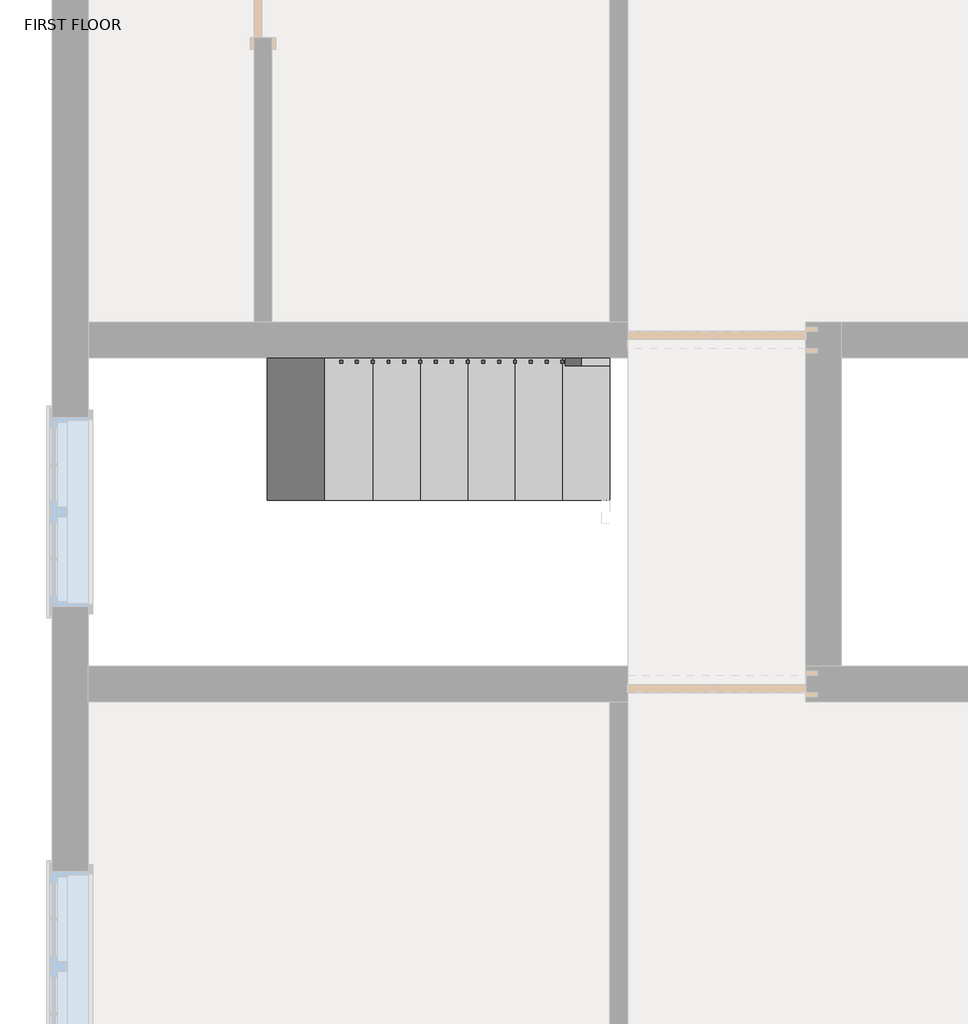
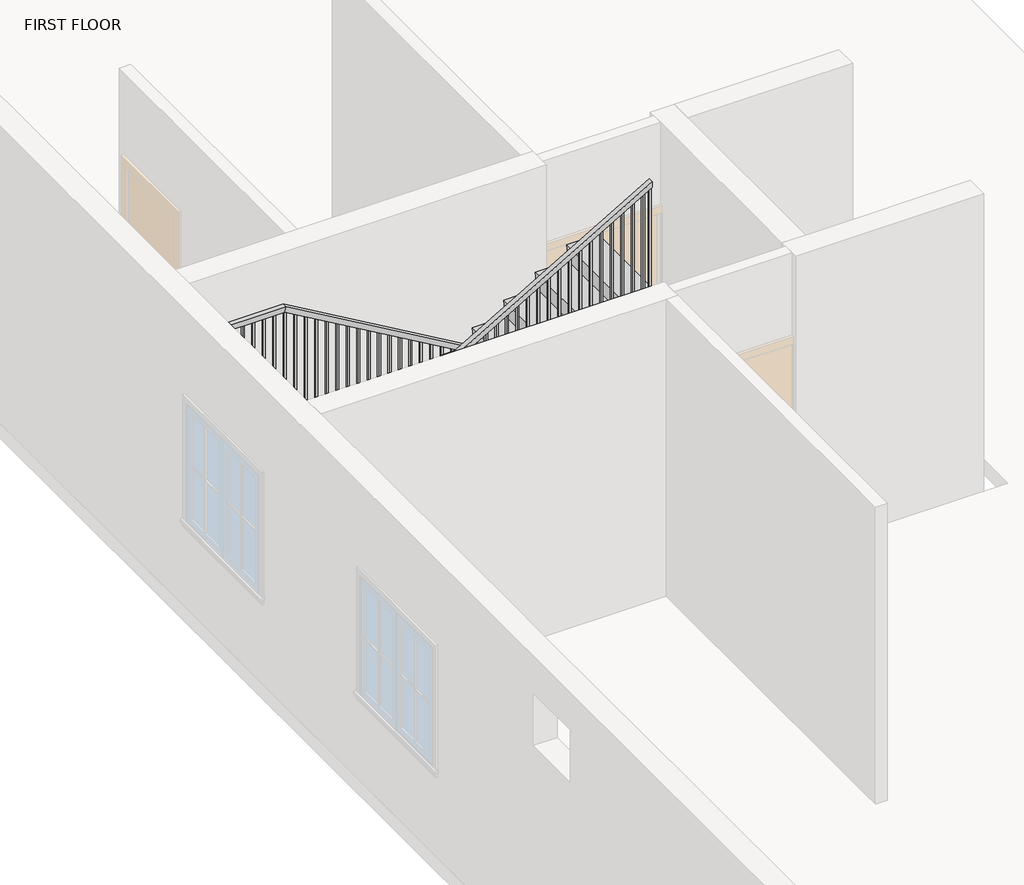
# One storey, part 3 of 4: 1 railing, 1 stair flight.
"""IFC4 building model written with IfcOpenShell, lengths in millimetres."""

from ifc_helpers import new_model, si_unit, frame, origin, place, context, project, spatial, polyline, outline, extrude, faceted_brep, element, save

model = new_model("IFC4")

# Units and contexts
model_context = context("Model", 3, world=origin())
ifc_project = project(units=[si_unit("LENGTHUNIT", "METRE", prefix="MILLI")], contexts=[model_context])

# Site, building, storey
site = spatial("IfcSite", under=ifc_project)
building = spatial("IfcBuilding", under=site)
storey = spatial("IfcBuildingStorey", under=building, Name="FIRST FLOOR", Elevation=3200.4)

# Railing
placement = place(None, origin())
element("IfcRailing", 1, ObjectType="Handrail - Rectangular", at=placement, inside=storey, context=model_context, shape_type="SolidModel", body=[
    faceted_brep([(-2776.8289041, 1499.0153263, 4292.6), (-2776.8289041, 1499.0153263, 4233.7886538), (-2776.8289041, 1549.8153263, 4233.7886538), (-2776.8289041, 1549.8153263, 4292.6), (-5215.2289041, 1499.0153263, 5715.0), (-5228.9626405, 1499.0153263, 5664.2), (-5228.9626405, 1549.8153263, 5664.2), (-5215.2289041, 1549.8153263, 5715.0), (-6078.8289041, 1499.0153263, 5715.0), (-6078.8289041, 1499.0153263, 5664.2), (-6129.6289041, 1549.8153263, 5664.2), (-6129.6289041, 1549.8153263, 5715.0), (-6078.8289041, -380.5846737, 5715.0), (-6078.8289041, -380.5846737, 5664.2), (-6129.6289041, -431.3846737, 5664.2), (-6129.6289041, -431.3846737, 5715.0), (-5520.0289041, -380.5846737, 5715.0), (-5506.2951677, -380.5846737, 5664.2), (-5506.2951677, -431.3846737, 5664.2), (-5520.0289041, -431.3846737, 5715.0), (-2776.8289041, -380.5846737, 7315.2), (-2776.8289041, -431.3846737, 7315.2), (-2776.8289041, -431.3846737, 7256.3886538), (-2776.8289041, -380.5846737, 7256.3886538)], [[[0, 1, 2, 3]], [[1, 0, 4, 5]], [[2, 1, 5, 6]], [[3, 2, 6, 7]], [[0, 3, 7, 4]], [[5, 4, 8, 9]], [[6, 5, 9, 10]], [[7, 6, 10, 11]], [[4, 7, 11, 8]], [[9, 8, 12, 13]], [[10, 9, 13, 14]], [[11, 10, 14, 15]], [[8, 11, 15, 12]], [[13, 12, 16, 17]], [[14, 13, 17, 18]], [[15, 14, 18, 19]], [[12, 15, 19, 16]], [[20, 21, 22, 23]], [[17, 16, 20, 23]], [[18, 17, 23, 22]], [[19, 18, 22, 21]], [[16, 19, 21, 20]]]),
    extrude(outline(polyline([(7217.4949038, -2843.5039041), (7206.3824038, -2862.5539041), (6223.0, -2862.5539041), (6223.0, -2843.5039041), (7217.4949038, -2843.5039041)])), frame((0.0, -415.5096737, 0.0), z_axis=(0.0, 1.0, 0.0), x_axis=(0.0, 0.0, 1.0)), (0.0, 0.0, 1.0), 19.05),
    extrude(outline(polyline([(7158.2282371, -2945.1039041), (7147.1157371, -2964.1539041), (6223.0, -2964.1539041), (6223.0, -2945.1039041), (7158.2282371, -2945.1039041)])), frame((0.0, -415.5096737, 0.0), z_axis=(0.0, 1.0, 0.0), x_axis=(0.0, 0.0, 1.0)), (0.0, 0.0, 1.0), 19.05),
    extrude(outline(polyline([(7098.9615704, -3046.7039041), (7087.8490704, -3065.7539041), (6223.0, -3065.7539041), (6223.0, -3046.7039041), (7098.9615704, -3046.7039041)])), frame((0.0, -415.5096737, 0.0), z_axis=(0.0, 1.0, 0.0), x_axis=(0.0, 0.0, 1.0)), (0.0, 0.0, 1.0), 19.05),
    extrude(outline(polyline([(7039.6949038, -3148.3039041), (7028.5824038, -3167.3539041), (6045.2, -3167.3539041), (6045.2, -3148.3039041), (7039.6949038, -3148.3039041)])), frame((0.0, -415.5096737, 0.0), z_axis=(0.0, 1.0, 0.0), x_axis=(0.0, 0.0, 1.0)), (0.0, 0.0, 1.0), 19.05),
    extrude(outline(polyline([(6980.4282371, -3249.9039041), (6969.3157371, -3268.9539041), (6045.2, -3268.9539041), (6045.2, -3249.9039041), (6980.4282371, -3249.9039041)])), frame((0.0, -415.5096737, 0.0), z_axis=(0.0, 1.0, 0.0), x_axis=(0.0, 0.0, 1.0)), (0.0, 0.0, 1.0), 19.05),
    extrude(outline(polyline([(6921.1615704, -3351.5039041), (6910.0490704, -3370.5539041), (6045.2, -3370.5539041), (6045.2, -3351.5039041), (6921.1615704, -3351.5039041)])), frame((0.0, -415.5096737, 0.0), z_axis=(0.0, 1.0, 0.0), x_axis=(0.0, 0.0, 1.0)), (0.0, 0.0, 1.0), 19.05),
    extrude(outline(polyline([(6861.8949038, -3453.1039041), (6850.7824038, -3472.1539041), (5867.4, -3472.1539041), (5867.4, -3453.1039041), (6861.8949038, -3453.1039041)])), frame((0.0, -415.5096737, 0.0), z_axis=(0.0, 1.0, 0.0), x_axis=(0.0, 0.0, 1.0)), (0.0, 0.0, 1.0), 19.05),
    extrude(outline(polyline([(6802.6282371, -3554.7039041), (6791.5157371, -3573.7539041), (5867.4, -3573.7539041), (5867.4, -3554.7039041), (6802.6282371, -3554.7039041)])), frame((0.0, -415.5096737, 0.0), z_axis=(0.0, 1.0, 0.0), x_axis=(0.0, 0.0, 1.0)), (0.0, 0.0, 1.0), 19.05),
    extrude(outline(polyline([(6743.3615704, -3656.3039041), (6732.2490704, -3675.3539041), (5867.4, -3675.3539041), (5867.4, -3656.3039041), (6743.3615704, -3656.3039041)])), frame((0.0, -415.5096737, 0.0), z_axis=(0.0, 1.0, 0.0), x_axis=(0.0, 0.0, 1.0)), (0.0, 0.0, 1.0), 19.05),
    extrude(outline(polyline([(6684.0949038, -3757.9039041), (6672.9824038, -3776.9539041), (5689.6, -3776.9539041), (5689.6, -3757.9039041), (6684.0949038, -3757.9039041)])), frame((0.0, -415.5096737, 0.0), z_axis=(0.0, 1.0, 0.0), x_axis=(0.0, 0.0, 1.0)), (0.0, 0.0, 1.0), 19.05),
    extrude(outline(polyline([(6624.8282371, -3859.5039041), (6613.7157371, -3878.5539041), (5689.6, -3878.5539041), (5689.6, -3859.5039041), (6624.8282371, -3859.5039041)])), frame((0.0, -415.5096737, 0.0), z_axis=(0.0, 1.0, 0.0), x_axis=(0.0, 0.0, 1.0)), (0.0, 0.0, 1.0), 19.05),
    extrude(outline(polyline([(6565.5615704, -3961.1039041), (6554.4490704, -3980.1539041), (5689.6, -3980.1539041), (5689.6, -3961.1039041), (6565.5615704, -3961.1039041)])), frame((0.0, -415.5096737, 0.0), z_axis=(0.0, 1.0, 0.0), x_axis=(0.0, 0.0, 1.0)), (0.0, 0.0, 1.0), 19.05),
    extrude(outline(polyline([(6506.2949038, -4062.7039041), (6495.1824038, -4081.7539041), (5511.8, -4081.7539041), (5511.8, -4062.7039041), (6506.2949038, -4062.7039041)])), frame((0.0, -415.5096737, 0.0), z_axis=(0.0, 1.0, 0.0), x_axis=(0.0, 0.0, 1.0)), (0.0, 0.0, 1.0), 19.05),
    extrude(outline(polyline([(6447.0282371, -4164.3039041), (6435.9157371, -4183.3539041), (5511.8, -4183.3539041), (5511.8, -4164.3039041), (6447.0282371, -4164.3039041)])), frame((0.0, -415.5096737, 0.0), z_axis=(0.0, 1.0, 0.0), x_axis=(0.0, 0.0, 1.0)), (0.0, 0.0, 1.0), 19.05),
    extrude(outline(polyline([(6387.7615704, -4265.9039041), (6376.6490704, -4284.9539041), (5511.8, -4284.9539041), (5511.8, -4265.9039041), (6387.7615704, -4265.9039041)])), frame((0.0, -415.5096737, 0.0), z_axis=(0.0, 1.0, 0.0), x_axis=(0.0, 0.0, 1.0)), (0.0, 0.0, 1.0), 19.05),
    extrude(outline(polyline([(6328.4949038, -4367.5039041), (6317.3824038, -4386.5539041), (5334.0, -4386.5539041), (5334.0, -4367.5039041), (6328.4949038, -4367.5039041)])), frame((0.0, -415.5096737, 0.0), z_axis=(0.0, 1.0, 0.0), x_axis=(0.0, 0.0, 1.0)), (0.0, 0.0, 1.0), 19.05),
    extrude(outline(polyline([(6269.2282371, -4469.1039041), (6258.1157371, -4488.1539041), (5334.0, -4488.1539041), (5334.0, -4469.1039041), (6269.2282371, -4469.1039041)])), frame((0.0, -415.5096737, 0.0), z_axis=(0.0, 1.0, 0.0), x_axis=(0.0, 0.0, 1.0)), (0.0, 0.0, 1.0), 19.05),
    extrude(outline(polyline([(6209.9615704, -4570.7039041), (6198.8490704, -4589.7539041), (5334.0, -4589.7539041), (5334.0, -4570.7039041), (6209.9615704, -4570.7039041)])), frame((0.0, -415.5096737, 0.0), z_axis=(0.0, 1.0, 0.0), x_axis=(0.0, 0.0, 1.0)), (0.0, 0.0, 1.0), 19.05),
    extrude(outline(polyline([(6150.6949038, -4672.3039041), (6139.5824038, -4691.3539041), (5156.2, -4691.3539041), (5156.2, -4672.3039041), (6150.6949038, -4672.3039041)])), frame((0.0, -415.5096737, 0.0), z_axis=(0.0, 1.0, 0.0), x_axis=(0.0, 0.0, 1.0)), (0.0, 0.0, 1.0), 19.05),
    extrude(outline(polyline([(6091.4282371, -4773.9039041), (6080.3157371, -4792.9539041), (5156.2, -4792.9539041), (5156.2, -4773.9039041), (6091.4282371, -4773.9039041)])), frame((0.0, -415.5096737, 0.0), z_axis=(0.0, 1.0, 0.0), x_axis=(0.0, 0.0, 1.0)), (0.0, 0.0, 1.0), 19.05),
    extrude(outline(polyline([(6032.1615704, -4875.5039041), (6021.0490704, -4894.5539041), (5156.2, -4894.5539041), (5156.2, -4875.5039041), (6032.1615704, -4875.5039041)])), frame((0.0, -415.5096737, 0.0), z_axis=(0.0, 1.0, 0.0), x_axis=(0.0, 0.0, 1.0)), (0.0, 0.0, 1.0), 19.05),
    extrude(outline(polyline([(5972.8949038, -4977.1039041), (5961.7824038, -4996.1539041), (4978.4, -4996.1539041), (4978.4, -4977.1039041), (5972.8949038, -4977.1039041)])), frame((0.0, -415.5096737, 0.0), z_axis=(0.0, 1.0, 0.0), x_axis=(0.0, 0.0, 1.0)), (0.0, 0.0, 1.0), 19.05),
    extrude(outline(polyline([(5913.6282371, -5078.7039041), (5902.5157371, -5097.7539041), (4978.4, -5097.7539041), (4978.4, -5078.7039041), (5913.6282371, -5078.7039041)])), frame((0.0, -415.5096737, 0.0), z_axis=(0.0, 1.0, 0.0), x_axis=(0.0, 0.0, 1.0)), (0.0, 0.0, 1.0), 19.05),
    extrude(outline(polyline([(5854.3615704, -5180.3039041), (5843.2490704, -5199.3539041), (4978.4, -5199.3539041), (4978.4, -5180.3039041), (5854.3615704, -5180.3039041)])), frame((0.0, -415.5096737, 0.0), z_axis=(0.0, 1.0, 0.0), x_axis=(0.0, 0.0, 1.0)), (0.0, 0.0, 1.0), 19.05),
    extrude(outline(polyline([(5795.0949038, -5281.9039041), (5783.9824038, -5300.9539041), (4800.6, -5300.9539041), (4800.6, -5281.9039041), (5795.0949038, -5281.9039041)])), frame((0.0, -415.5096737, 0.0), z_axis=(0.0, 1.0, 0.0), x_axis=(0.0, 0.0, 1.0)), (0.0, 0.0, 1.0), 19.05),
    extrude(outline(polyline([(5735.8282371, -5383.5039041), (5724.7157371, -5402.5539041), (4800.6, -5402.5539041), (4800.6, -5383.5039041), (5735.8282371, -5383.5039041)])), frame((0.0, -415.5096737, 0.0), z_axis=(0.0, 1.0, 0.0), x_axis=(0.0, 0.0, 1.0)), (0.0, 0.0, 1.0), 19.05),
    extrude(outline(polyline([(5676.5615704, -5485.1039041), (5665.4490704, -5504.1539041), (4800.6, -5504.1539041), (4800.6, -5485.1039041), (5676.5615704, -5485.1039041)])), frame((0.0, -415.5096737, 0.0), z_axis=(0.0, 1.0, 0.0), x_axis=(0.0, 0.0, 1.0)), (0.0, 0.0, 1.0), 19.05),
    extrude(outline(polyline([(-5605.7539041, -415.5096737), (-5605.7539041, -396.4596737), (-5586.7039041, -396.4596737), (-5586.7039041, -415.5096737), (-5605.7539041, -415.5096737)])), frame((0.0, 0.0, 4800.6), z_axis=(0.0, 0.0, 1.0), x_axis=(1.0, 0.0, 0.0)), (0.0, 0.0, 1.0), 863.6),
    extrude(outline(polyline([(-5707.3539041, -415.5096737), (-5707.3539041, -396.4596737), (-5688.3039041, -396.4596737), (-5688.3039041, -415.5096737), (-5707.3539041, -415.5096737)])), frame((0.0, 0.0, 4800.6), z_axis=(0.0, 0.0, 1.0), x_axis=(1.0, 0.0, 0.0)), (0.0, 0.0, 1.0), 863.6),
    extrude(outline(polyline([(-5808.9539041, -415.5096737), (-5808.9539041, -396.4596737), (-5789.9039041, -396.4596737), (-5789.9039041, -415.5096737), (-5808.9539041, -415.5096737)])), frame((0.0, 0.0, 4800.6), z_axis=(0.0, 0.0, 1.0), x_axis=(1.0, 0.0, 0.0)), (0.0, 0.0, 1.0), 863.6),
    extrude(outline(polyline([(-5910.5539041, -415.5096737), (-5910.5539041, -396.4596737), (-5891.5039041, -396.4596737), (-5891.5039041, -415.5096737), (-5910.5539041, -415.5096737)])), frame((0.0, 0.0, 4800.6), z_axis=(0.0, 0.0, 1.0), x_axis=(1.0, 0.0, 0.0)), (0.0, 0.0, 1.0), 863.6),
    extrude(outline(polyline([(-6012.1539041, -415.5096737), (-6012.1539041, -396.4596737), (-5993.1039041, -396.4596737), (-5993.1039041, -415.5096737), (-6012.1539041, -415.5096737)])), frame((0.0, 0.0, 4800.6), z_axis=(0.0, 0.0, 1.0), x_axis=(1.0, 0.0, 0.0)), (0.0, 0.0, 1.0), 863.6),
    extrude(outline(polyline([(-6113.7539041, -294.8596737), (-6094.7039041, -294.8596737), (-6094.7039041, -313.9096737), (-6113.7539041, -313.9096737), (-6113.7539041, -294.8596737)])), frame((0.0, 0.0, 4800.6), z_axis=(0.0, 0.0, 1.0), x_axis=(1.0, 0.0, 0.0)), (0.0, 0.0, 1.0), 863.6),
    extrude(outline(polyline([(-6113.7539041, -193.2596737), (-6094.7039041, -193.2596737), (-6094.7039041, -212.3096737), (-6113.7539041, -212.3096737), (-6113.7539041, -193.2596737)])), frame((0.0, 0.0, 4800.6), z_axis=(0.0, 0.0, 1.0), x_axis=(1.0, 0.0, 0.0)), (0.0, 0.0, 1.0), 863.6),
    extrude(outline(polyline([(-6113.7539041, -91.6596737), (-6094.7039041, -91.6596737), (-6094.7039041, -110.7096737), (-6113.7539041, -110.7096737), (-6113.7539041, -91.6596737)])), frame((0.0, 0.0, 4800.6), z_axis=(0.0, 0.0, 1.0), x_axis=(1.0, 0.0, 0.0)), (0.0, 0.0, 1.0), 863.6),
    extrude(outline(polyline([(-6113.7539041, 9.9403263), (-6094.7039041, 9.9403263), (-6094.7039041, -9.1096737), (-6113.7539041, -9.1096737), (-6113.7539041, 9.9403263)])), frame((0.0, 0.0, 4800.6), z_axis=(0.0, 0.0, 1.0), x_axis=(1.0, 0.0, 0.0)), (0.0, 0.0, 1.0), 863.6),
    extrude(outline(polyline([(-6113.7539041, 111.5403263), (-6094.7039041, 111.5403263), (-6094.7039041, 92.4903263), (-6113.7539041, 92.4903263), (-6113.7539041, 111.5403263)])), frame((0.0, 0.0, 4800.6), z_axis=(0.0, 0.0, 1.0), x_axis=(1.0, 0.0, 0.0)), (0.0, 0.0, 1.0), 863.6),
    extrude(outline(polyline([(-6113.7539041, 213.1403263), (-6094.7039041, 213.1403263), (-6094.7039041, 194.0903263), (-6113.7539041, 194.0903263), (-6113.7539041, 213.1403263)])), frame((0.0, 0.0, 4800.6), z_axis=(0.0, 0.0, 1.0), x_axis=(1.0, 0.0, 0.0)), (0.0, 0.0, 1.0), 863.6),
    extrude(outline(polyline([(-6113.7539041, 314.7403263), (-6094.7039041, 314.7403263), (-6094.7039041, 295.6903263), (-6113.7539041, 295.6903263), (-6113.7539041, 314.7403263)])), frame((0.0, 0.0, 4800.6), z_axis=(0.0, 0.0, 1.0), x_axis=(1.0, 0.0, 0.0)), (0.0, 0.0, 1.0), 863.6),
    extrude(outline(polyline([(-6113.7539041, 416.3403263), (-6094.7039041, 416.3403263), (-6094.7039041, 397.2903263), (-6113.7539041, 397.2903263), (-6113.7539041, 416.3403263)])), frame((0.0, 0.0, 4800.6), z_axis=(0.0, 0.0, 1.0), x_axis=(1.0, 0.0, 0.0)), (0.0, 0.0, 1.0), 863.6),
    extrude(outline(polyline([(-6113.7539041, 517.9403263), (-6094.7039041, 517.9403263), (-6094.7039041, 498.8903263), (-6113.7539041, 498.8903263), (-6113.7539041, 517.9403263)])), frame((0.0, 0.0, 4800.6), z_axis=(0.0, 0.0, 1.0), x_axis=(1.0, 0.0, 0.0)), (0.0, 0.0, 1.0), 863.6),
    extrude(outline(polyline([(-6113.7539041, 619.5403263), (-6094.7039041, 619.5403263), (-6094.7039041, 600.4903263), (-6113.7539041, 600.4903263), (-6113.7539041, 619.5403263)])), frame((0.0, 0.0, 4800.6), z_axis=(0.0, 0.0, 1.0), x_axis=(1.0, 0.0, 0.0)), (0.0, 0.0, 1.0), 863.6),
    extrude(outline(polyline([(-6113.7539041, 721.1403263), (-6094.7039041, 721.1403263), (-6094.7039041, 702.0903263), (-6113.7539041, 702.0903263), (-6113.7539041, 721.1403263)])), frame((0.0, 0.0, 4800.6), z_axis=(0.0, 0.0, 1.0), x_axis=(1.0, 0.0, 0.0)), (0.0, 0.0, 1.0), 863.6),
    extrude(outline(polyline([(-6113.7539041, 822.7403263), (-6094.7039041, 822.7403263), (-6094.7039041, 803.6903263), (-6113.7539041, 803.6903263), (-6113.7539041, 822.7403263)])), frame((0.0, 0.0, 4800.6), z_axis=(0.0, 0.0, 1.0), x_axis=(1.0, 0.0, 0.0)), (0.0, 0.0, 1.0), 863.6),
    extrude(outline(polyline([(-6113.7539041, 924.3403263), (-6094.7039041, 924.3403263), (-6094.7039041, 905.2903263), (-6113.7539041, 905.2903263), (-6113.7539041, 924.3403263)])), frame((0.0, 0.0, 4800.6), z_axis=(0.0, 0.0, 1.0), x_axis=(1.0, 0.0, 0.0)), (0.0, 0.0, 1.0), 863.6),
    extrude(outline(polyline([(-6113.7539041, 1025.9403263), (-6094.7039041, 1025.9403263), (-6094.7039041, 1006.8903263), (-6113.7539041, 1006.8903263), (-6113.7539041, 1025.9403263)])), frame((0.0, 0.0, 4800.6), z_axis=(0.0, 0.0, 1.0), x_axis=(1.0, 0.0, 0.0)), (0.0, 0.0, 1.0), 863.6),
    extrude(outline(polyline([(-6113.7539041, 1127.5403263), (-6094.7039041, 1127.5403263), (-6094.7039041, 1108.4903263), (-6113.7539041, 1108.4903263), (-6113.7539041, 1127.5403263)])), frame((0.0, 0.0, 4800.6), z_axis=(0.0, 0.0, 1.0), x_axis=(1.0, 0.0, 0.0)), (0.0, 0.0, 1.0), 863.6),
    extrude(outline(polyline([(-6113.7539041, 1229.1403263), (-6094.7039041, 1229.1403263), (-6094.7039041, 1210.0903263), (-6113.7539041, 1210.0903263), (-6113.7539041, 1229.1403263)])), frame((0.0, 0.0, 4800.6), z_axis=(0.0, 0.0, 1.0), x_axis=(1.0, 0.0, 0.0)), (0.0, 0.0, 1.0), 863.6),
    extrude(outline(polyline([(-6113.7539041, 1330.7403263), (-6094.7039041, 1330.7403263), (-6094.7039041, 1311.6903263), (-6113.7539041, 1311.6903263), (-6113.7539041, 1330.7403263)])), frame((0.0, 0.0, 4800.6), z_axis=(0.0, 0.0, 1.0), x_axis=(1.0, 0.0, 0.0)), (0.0, 0.0, 1.0), 863.6),
    extrude(outline(polyline([(-6113.7539041, 1432.3403263), (-6094.7039041, 1432.3403263), (-6094.7039041, 1413.2903263), (-6113.7539041, 1413.2903263), (-6113.7539041, 1432.3403263)])), frame((0.0, 0.0, 4800.6), z_axis=(0.0, 0.0, 1.0), x_axis=(1.0, 0.0, 0.0)), (0.0, 0.0, 1.0), 863.6),
    extrude(outline(polyline([(-6018.5039041, 1533.9403263), (-6018.5039041, 1514.8903263), (-6037.5539041, 1514.8903263), (-6037.5539041, 1533.9403263), (-6018.5039041, 1533.9403263)])), frame((0.0, 0.0, 4800.6), z_axis=(0.0, 0.0, 1.0), x_axis=(1.0, 0.0, 0.0)), (0.0, 0.0, 1.0), 863.6),
    extrude(outline(polyline([(-5916.9039041, 1533.9403263), (-5916.9039041, 1514.8903263), (-5935.9539041, 1514.8903263), (-5935.9539041, 1533.9403263), (-5916.9039041, 1533.9403263)])), frame((0.0, 0.0, 4800.6), z_axis=(0.0, 0.0, 1.0), x_axis=(1.0, 0.0, 0.0)), (0.0, 0.0, 1.0), 863.6),
    extrude(outline(polyline([(-5815.3039041, 1533.9403263), (-5815.3039041, 1514.8903263), (-5834.3539041, 1514.8903263), (-5834.3539041, 1533.9403263), (-5815.3039041, 1533.9403263)])), frame((0.0, 0.0, 4800.6), z_axis=(0.0, 0.0, 1.0), x_axis=(1.0, 0.0, 0.0)), (0.0, 0.0, 1.0), 863.6),
    extrude(outline(polyline([(-5713.7039041, 1533.9403263), (-5713.7039041, 1514.8903263), (-5732.7539041, 1514.8903263), (-5732.7539041, 1533.9403263), (-5713.7039041, 1533.9403263)])), frame((0.0, 0.0, 4800.6), z_axis=(0.0, 0.0, 1.0), x_axis=(1.0, 0.0, 0.0)), (0.0, 0.0, 1.0), 863.6),
    extrude(outline(polyline([(-5612.1039041, 1533.9403263), (-5612.1039041, 1514.8903263), (-5631.1539041, 1514.8903263), (-5631.1539041, 1533.9403263), (-5612.1039041, 1533.9403263)])), frame((0.0, 0.0, 4800.6), z_axis=(0.0, 0.0, 1.0), x_axis=(1.0, 0.0, 0.0)), (0.0, 0.0, 1.0), 863.6),
    extrude(outline(polyline([(-5510.5039041, 1533.9403263), (-5510.5039041, 1514.8903263), (-5529.5539041, 1514.8903263), (-5529.5539041, 1533.9403263), (-5510.5039041, 1533.9403263)])), frame((0.0, 0.0, 4800.6), z_axis=(0.0, 0.0, 1.0), x_axis=(1.0, 0.0, 0.0)), (0.0, 0.0, 1.0), 863.6),
    extrude(outline(polyline([(-5408.9039041, 1533.9403263), (-5408.9039041, 1514.8903263), (-5427.9539041, 1514.8903263), (-5427.9539041, 1533.9403263), (-5408.9039041, 1533.9403263)])), frame((0.0, 0.0, 4800.6), z_axis=(0.0, 0.0, 1.0), x_axis=(1.0, 0.0, 0.0)), (0.0, 0.0, 1.0), 863.6),
    extrude(outline(polyline([(-5307.3039041, 1533.9403263), (-5307.3039041, 1514.8903263), (-5326.3539041, 1514.8903263), (-5326.3539041, 1533.9403263), (-5307.3039041, 1533.9403263)])), frame((0.0, 0.0, 4800.6), z_axis=(0.0, 0.0, 1.0), x_axis=(1.0, 0.0, 0.0)), (0.0, 0.0, 1.0), 863.6),
    extrude(outline(polyline([(5650.6324038, -5205.7039041), (5661.7449038, -5224.7539041), (4800.6, -5224.7539041), (4800.6, -5205.7039041), (5650.6324038, -5205.7039041)])), frame((0.0, 1514.8903263, 0.0), z_axis=(0.0, 1.0, 0.0), x_axis=(0.0, 0.0, 1.0)), (0.0, 0.0, 1.0), 19.05),
    extrude(outline(polyline([(5591.3657371, -5104.1039041), (5602.4782371, -5123.1539041), (4622.8, -5123.1539041), (4622.8, -5104.1039041), (5591.3657371, -5104.1039041)])), frame((0.0, 1514.8903263, 0.0), z_axis=(0.0, 1.0, 0.0), x_axis=(0.0, 0.0, 1.0)), (0.0, 0.0, 1.0), 19.05),
    extrude(outline(polyline([(5532.0990704, -5002.5039041), (5543.2115704, -5021.5539041), (4622.8, -5021.5539041), (4622.8, -5002.5039041), (5532.0990704, -5002.5039041)])), frame((0.0, 1514.8903263, 0.0), z_axis=(0.0, 1.0, 0.0), x_axis=(0.0, 0.0, 1.0)), (0.0, 0.0, 1.0), 19.05),
    extrude(outline(polyline([(5472.8324038, -4900.9039041), (5483.9449038, -4919.9539041), (4622.8, -4919.9539041), (4622.8, -4900.9039041), (5472.8324038, -4900.9039041)])), frame((0.0, 1514.8903263, 0.0), z_axis=(0.0, 1.0, 0.0), x_axis=(0.0, 0.0, 1.0)), (0.0, 0.0, 1.0), 19.05),
    extrude(outline(polyline([(5413.5657371, -4799.3039041), (5424.6782371, -4818.3539041), (4445.0, -4818.3539041), (4445.0, -4799.3039041), (5413.5657371, -4799.3039041)])), frame((0.0, 1514.8903263, 0.0), z_axis=(0.0, 1.0, 0.0), x_axis=(0.0, 0.0, 1.0)), (0.0, 0.0, 1.0), 19.05),
    extrude(outline(polyline([(5354.2990704, -4697.7039041), (5365.4115704, -4716.7539041), (4445.0, -4716.7539041), (4445.0, -4697.7039041), (5354.2990704, -4697.7039041)])), frame((0.0, 1514.8903263, 0.0), z_axis=(0.0, 1.0, 0.0), x_axis=(0.0, 0.0, 1.0)), (0.0, 0.0, 1.0), 19.05),
    extrude(outline(polyline([(5295.0324038, -4596.1039041), (5306.1449038, -4615.1539041), (4445.0, -4615.1539041), (4445.0, -4596.1039041), (5295.0324038, -4596.1039041)])), frame((0.0, 1514.8903263, 0.0), z_axis=(0.0, 1.0, 0.0), x_axis=(0.0, 0.0, 1.0)), (0.0, 0.0, 1.0), 19.05),
    extrude(outline(polyline([(5235.7657371, -4494.5039041), (5246.8782371, -4513.5539041), (4267.2, -4513.5539041), (4267.2, -4494.5039041), (5235.7657371, -4494.5039041)])), frame((0.0, 1514.8903263, 0.0), z_axis=(0.0, 1.0, 0.0), x_axis=(0.0, 0.0, 1.0)), (0.0, 0.0, 1.0), 19.05),
    extrude(outline(polyline([(5176.4990704, -4392.9039041), (5187.6115704, -4411.9539041), (4267.2, -4411.9539041), (4267.2, -4392.9039041), (5176.4990704, -4392.9039041)])), frame((0.0, 1514.8903263, 0.0), z_axis=(0.0, 1.0, 0.0), x_axis=(0.0, 0.0, 1.0)), (0.0, 0.0, 1.0), 19.05),
    extrude(outline(polyline([(5117.2324038, -4291.3039041), (5128.3449038, -4310.3539041), (4267.2, -4310.3539041), (4267.2, -4291.3039041), (5117.2324038, -4291.3039041)])), frame((0.0, 1514.8903263, 0.0), z_axis=(0.0, 1.0, 0.0), x_axis=(0.0, 0.0, 1.0)), (0.0, 0.0, 1.0), 19.05),
    extrude(outline(polyline([(5057.9657371, -4189.7039041), (5069.0782371, -4208.7539041), (4089.4, -4208.7539041), (4089.4, -4189.7039041), (5057.9657371, -4189.7039041)])), frame((0.0, 1514.8903263, 0.0), z_axis=(0.0, 1.0, 0.0), x_axis=(0.0, 0.0, 1.0)), (0.0, 0.0, 1.0), 19.05),
    extrude(outline(polyline([(4998.6990704, -4088.1039041), (5009.8115704, -4107.1539041), (4089.4, -4107.1539041), (4089.4, -4088.1039041), (4998.6990704, -4088.1039041)])), frame((0.0, 1514.8903263, 0.0), z_axis=(0.0, 1.0, 0.0), x_axis=(0.0, 0.0, 1.0)), (0.0, 0.0, 1.0), 19.05),
    extrude(outline(polyline([(4939.4324038, -3986.5039041), (4950.5449038, -4005.5539041), (4089.4, -4005.5539041), (4089.4, -3986.5039041), (4939.4324038, -3986.5039041)])), frame((0.0, 1514.8903263, 0.0), z_axis=(0.0, 1.0, 0.0), x_axis=(0.0, 0.0, 1.0)), (0.0, 0.0, 1.0), 19.05),
    extrude(outline(polyline([(4880.1657371, -3884.9039041), (4891.2782371, -3903.9539041), (3911.6, -3903.9539041), (3911.6, -3884.9039041), (4880.1657371, -3884.9039041)])), frame((0.0, 1514.8903263, 0.0), z_axis=(0.0, 1.0, 0.0), x_axis=(0.0, 0.0, 1.0)), (0.0, 0.0, 1.0), 19.05),
    extrude(outline(polyline([(4820.8990704, -3783.3039041), (4832.0115704, -3802.3539041), (3911.6, -3802.3539041), (3911.6, -3783.3039041), (4820.8990704, -3783.3039041)])), frame((0.0, 1514.8903263, 0.0), z_axis=(0.0, 1.0, 0.0), x_axis=(0.0, 0.0, 1.0)), (0.0, 0.0, 1.0), 19.05),
    extrude(outline(polyline([(4761.6324038, -3681.7039041), (4772.7449038, -3700.7539041), (3911.6, -3700.7539041), (3911.6, -3681.7039041), (4761.6324038, -3681.7039041)])), frame((0.0, 1514.8903263, 0.0), z_axis=(0.0, 1.0, 0.0), x_axis=(0.0, 0.0, 1.0)), (0.0, 0.0, 1.0), 19.05),
    extrude(outline(polyline([(4702.3657371, -3580.1039041), (4713.4782371, -3599.1539041), (3733.8, -3599.1539041), (3733.8, -3580.1039041), (4702.3657371, -3580.1039041)])), frame((0.0, 1514.8903263, 0.0), z_axis=(0.0, 1.0, 0.0), x_axis=(0.0, 0.0, 1.0)), (0.0, 0.0, 1.0), 19.05),
    extrude(outline(polyline([(4643.0990704, -3478.5039041), (4654.2115704, -3497.5539041), (3733.8, -3497.5539041), (3733.8, -3478.5039041), (4643.0990704, -3478.5039041)])), frame((0.0, 1514.8903263, 0.0), z_axis=(0.0, 1.0, 0.0), x_axis=(0.0, 0.0, 1.0)), (0.0, 0.0, 1.0), 19.05),
    extrude(outline(polyline([(4583.8324038, -3376.9039041), (4594.9449038, -3395.9539041), (3733.8, -3395.9539041), (3733.8, -3376.9039041), (4583.8324038, -3376.9039041)])), frame((0.0, 1514.8903263, 0.0), z_axis=(0.0, 1.0, 0.0), x_axis=(0.0, 0.0, 1.0)), (0.0, 0.0, 1.0), 19.05),
    extrude(outline(polyline([(4524.5657371, -3275.3039041), (4535.6782371, -3294.3539041), (3556.0, -3294.3539041), (3556.0, -3275.3039041), (4524.5657371, -3275.3039041)])), frame((0.0, 1514.8903263, 0.0), z_axis=(0.0, 1.0, 0.0), x_axis=(0.0, 0.0, 1.0)), (0.0, 0.0, 1.0), 19.05),
    extrude(outline(polyline([(4465.2990704, -3173.7039041), (4476.4115704, -3192.7539041), (3556.0, -3192.7539041), (3556.0, -3173.7039041), (4465.2990704, -3173.7039041)])), frame((0.0, 1514.8903263, 0.0), z_axis=(0.0, 1.0, 0.0), x_axis=(0.0, 0.0, 1.0)), (0.0, 0.0, 1.0), 19.05),
    extrude(outline(polyline([(4406.0324038, -3072.1039041), (4417.1449038, -3091.1539041), (3556.0, -3091.1539041), (3556.0, -3072.1039041), (4406.0324038, -3072.1039041)])), frame((0.0, 1514.8903263, 0.0), z_axis=(0.0, 1.0, 0.0), x_axis=(0.0, 0.0, 1.0)), (0.0, 0.0, 1.0), 19.05),
    extrude(outline(polyline([(4346.7657371, -2970.5039041), (4357.8782371, -2989.5539041), (3378.2, -2989.5539041), (3378.2, -2970.5039041), (4346.7657371, -2970.5039041)])), frame((0.0, 1514.8903263, 0.0), z_axis=(0.0, 1.0, 0.0), x_axis=(0.0, 0.0, 1.0)), (0.0, 0.0, 1.0), 19.05),
    extrude(outline(polyline([(4287.4990704, -2868.9039041), (4298.6115704, -2887.9539041), (3378.2, -2887.9539041), (3378.2, -2868.9039041), (4287.4990704, -2868.9039041)])), frame((0.0, 1514.8903263, 0.0), z_axis=(0.0, 1.0, 0.0), x_axis=(0.0, 0.0, 1.0)), (0.0, 0.0, 1.0), 19.05),
    extrude(outline(polyline([(-6113.7539041, -396.4596737), (-6094.7039041, -396.4596737), (-6094.7039041, -415.5096737), (-6113.7539041, -415.5096737), (-6113.7539041, -396.4596737)])), frame((0.0, 0.0, 4800.6), z_axis=(0.0, 0.0, 1.0), x_axis=(1.0, 0.0, 0.0)), (0.0, 0.0, 1.0), 863.6),
    extrude(outline(polyline([(-6094.7039041, 1533.9403263), (-6094.7039041, 1514.8903263), (-6113.7539041, 1514.8903263), (-6113.7539041, 1533.9403263), (-6094.7039041, 1533.9403263)])), frame((0.0, 0.0, 4800.6), z_axis=(0.0, 0.0, 1.0), x_axis=(1.0, 0.0, 0.0)), (0.0, 0.0, 1.0), 863.6),
    extrude(outline(polyline([(7256.3886538, -2776.8289041), (7245.2761538, -2795.8789041), (6223.0, -2795.8789041), (6223.0, -2776.8289041), (7256.3886538, -2776.8289041)])), frame((0.0, -415.5096737, 0.0), z_axis=(0.0, 1.0, 0.0), x_axis=(0.0, 0.0, 1.0)), (0.0, 0.0, 1.0), 19.05),
    extrude(outline(polyline([(4233.7886538, -2776.8289041), (4244.9011538, -2795.8789041), (3378.2, -2795.8789041), (3378.2, -2776.8289041), (4233.7886538, -2776.8289041)])), frame((0.0, 1514.8903263, 0.0), z_axis=(0.0, 1.0, 0.0), x_axis=(0.0, 0.0, 1.0)), (0.0, 0.0, 1.0), 19.05),
])

# Stair flight
element("IfcStairFlight", 2, ObjectType="3/4\" Nosing", at=placement, inside=storey, context=model_context, shape_type="Brep", body=[
    faceted_brep([(-2776.8289041, 635.4153263, 3378.2), (-2776.8289041, 1549.8153263, 3378.2), (-3100.6789041, 1549.8153263, 3378.2), (-3100.6789041, 635.4153263, 3378.2), (-3100.6789041, 635.4153263, 3304.6858172), (-2921.9032174, 635.4153263, 3200.4), (-2795.8789041, 635.4153263, 3200.4), (-2795.8789041, 1549.8153263, 3200.4), (-2921.9032174, 1549.8153263, 3200.4), (-3100.6789041, 1549.8153263, 3304.6858172), (-3081.6289041, 635.4153263, 3556.0), (-3081.6289041, 1549.8153263, 3556.0), (-3405.4789041, 1549.8153263, 3556.0), (-3405.4789041, 635.4153263, 3556.0), (-3405.4789041, 635.4153263, 3482.4858172), (-3405.4789041, 1549.8153263, 3482.4858172), (-3386.4289041, 635.4153263, 3733.8), (-3386.4289041, 1549.8153263, 3733.8), (-3710.2789041, 1549.8153263, 3733.8), (-3710.2789041, 635.4153263, 3733.8), (-3710.2789041, 635.4153263, 3660.2858172), (-3710.2789041, 1549.8153263, 3660.2858172), (-3691.2289041, 635.4153263, 3911.6), (-3691.2289041, 1549.8153263, 3911.6), (-4015.0789041, 1549.8153263, 3911.6), (-4015.0789041, 635.4153263, 3911.6), (-4015.0789041, 635.4153263, 3838.0858172), (-4015.0789041, 1549.8153263, 3838.0858172), (-3996.0289041, 635.4153263, 4089.4), (-3996.0289041, 1549.8153263, 4089.4), (-4319.8789041, 1549.8153263, 4089.4), (-4319.8789041, 635.4153263, 4089.4), (-4300.8289041, 635.4153263, 4267.2), (-4624.6789041, 635.4153263, 4267.2), (-4605.6289041, 635.4153263, 4445.0), (-4929.4789041, 635.4153263, 4445.0), (-4910.4289041, 635.4153263, 4622.8), (-5234.2789041, 635.4153263, 4622.8), (-5222.0324755, 635.4153263, 4737.1), (-5556.2460745, 635.4153263, 4737.1), (-4319.8789041, 1549.8153263, 4015.8858172), (-4300.8289041, 1549.8153263, 4267.2), (-4624.6789041, 1549.8153263, 4267.2), (-4624.6789041, 1549.8153263, 4193.6858172), (-4605.6289041, 1549.8153263, 4445.0), (-4929.4789041, 1549.8153263, 4445.0), (-4929.4789041, 1549.8153263, 4371.4858172), (-4910.4289041, 1549.8153263, 4622.8), (-5234.2789041, 1549.8153263, 4622.8), (-5234.2789041, 1549.8153263, 4549.2858172), (-5070.1545907, 483.0153263, 4800.6), (-2776.8289041, 483.0153263, 4800.6), (-2776.8289041, 635.4153263, 4800.6), (-3836.3032174, 635.4153263, 4800.6), (-5215.2289041, 635.4153263, 4800.6), (-5215.2289041, 1549.8153263, 4800.6), (-5556.2460745, 1549.8153263, 4800.6), (-6129.6289041, 1549.8153263, 4800.6), (-6129.6289041, -431.3846737, 4800.6), (-5196.1789041, -431.3846737, 4800.6), (-5196.1789041, 483.0153263, 4800.6), (-5179.0117336, 483.0153263, 4737.1), (-2776.8289041, 483.0153263, 4737.1), (-2776.8289041, 635.4153263, 4737.1), (-3727.4460745, 635.4153263, 4737.1), (-5556.2460745, 1549.8153263, 4737.1), (-6129.6289041, 1549.8153263, 4737.1), (-6129.6289041, -431.3846737, 4737.1), (-5196.1789041, -431.3846737, 4737.1), (-5215.2289041, 483.0153263, 4978.4), (-5215.2289041, -431.3846737, 4978.4), (-5179.0117336, -431.3846737, 4978.4), (-4891.3789041, -431.3846737, 4978.4), (-4891.3789041, 483.0153263, 4978.4), (-4891.3789041, 483.0153263, 4904.8858172), (-5179.0117336, -431.3846737, 4737.1), (-4891.3789041, -431.3846737, 4904.8858172), (-4910.4289041, 483.0153263, 5156.2), (-4910.4289041, -431.3846737, 5156.2), (-4586.5789041, -431.3846737, 5156.2), (-4586.5789041, 483.0153263, 5156.2), (-4586.5789041, 483.0153263, 5082.6858172), (-4586.5789041, -431.3846737, 5082.6858172), (-4605.6289041, 483.0153263, 5334.0), (-4605.6289041, -431.3846737, 5334.0), (-4281.7789041, -431.3846737, 5334.0), (-4281.7789041, 483.0153263, 5334.0), (-4281.7789041, 483.0153263, 5270.5), (-4281.7789041, 483.0153263, 5260.4858172), (-4598.8253326, 483.0153263, 5270.5), (-4281.7789041, -431.3846737, 5260.4858172), (-4300.8289041, 483.0153263, 5511.8), (-4300.8289041, -431.3846737, 5511.8), (-3976.9789041, -431.3846737, 5511.8), (-3976.9789041, 483.0153263, 5511.8), (-3976.9789041, 483.0153263, 5438.2858172), (-4264.6117336, 483.0153263, 5270.5), (-3976.9789041, -431.3846737, 5438.2858172), (-3996.0289041, 483.0153263, 5689.6), (-3996.0289041, -431.3846737, 5689.6), (-3672.1789041, -431.3846737, 5689.6), (-3672.1789041, 483.0153263, 5689.6), (-3672.1789041, 483.0153263, 5616.0858172), (-3672.1789041, -431.3846737, 5616.0858172), (-3691.2289041, 483.0153263, 5867.4), (-3691.2289041, -431.3846737, 5867.4), (-3367.3789041, -431.3846737, 5867.4), (-3367.3789041, 483.0153263, 5867.4), (-3367.3789041, 483.0153263, 5793.8858172), (-3367.3789041, -431.3846737, 5793.8858172), (-3386.4289041, 483.0153263, 6045.2), (-3386.4289041, -431.3846737, 6045.2), (-3062.5789041, -431.3846737, 6045.2), (-3062.5789041, 483.0153263, 6045.2), (-3062.5789041, 483.0153263, 5971.6858172), (-3062.5789041, -431.3846737, 5971.6858172), (-3081.6289041, 483.0153263, 6223.0), (-3081.6289041, -431.3846737, 6223.0), (-2776.8289041, -431.3846737, 6223.0), (-2776.8289041, 483.0153263, 6223.0), (-2776.8289041, 483.0153263, 6138.3733172), (-2776.8289041, -431.3846737, 6138.3733172)], [[[0, 1, 2, 3]], [[0, 3, 4, 5, 6]], [[2, 1, 7, 8, 9]], [[10, 11, 12, 13]], [[10, 13, 14, 4, 3]], [[12, 11, 2, 9, 15]], [[16, 17, 18, 19]], [[16, 19, 20, 14, 13]], [[18, 17, 12, 15, 21]], [[22, 23, 24, 25]], [[22, 25, 26, 20, 19]], [[24, 23, 18, 21, 27]], [[28, 29, 30, 31]], [[26, 25, 28, 31, 32, 33, 34, 35, 36, 37, 38, 39]], [[30, 29, 24, 27, 40]], [[32, 41, 42, 33]], [[42, 41, 30, 40, 43]], [[34, 44, 45, 35]], [[45, 44, 42, 43, 46]], [[36, 47, 48, 37]], [[48, 47, 45, 46, 49]], [[50, 51, 52, 53, 54, 55, 56, 57, 58, 59, 60]], [[50, 61, 62, 51]], [[52, 51, 62, 63]], [[52, 63, 64, 38, 54, 53]], [[55, 48, 49, 65, 66, 57, 56]], [[58, 57, 66, 67]], [[59, 58, 67, 68]], [[69, 70, 71, 72, 73]], [[69, 73, 74, 50, 60]], [[70, 59, 68, 75, 76, 72, 71]], [[77, 78, 79, 80]], [[77, 80, 81, 74, 73]], [[79, 78, 72, 76, 82]], [[83, 84, 85, 86]], [[83, 86, 87, 88, 81, 80, 89]], [[85, 84, 79, 82, 90]], [[91, 92, 93, 94]], [[91, 94, 95, 96, 88, 87, 86]], [[93, 92, 85, 90, 97]], [[98, 99, 100, 101]], [[98, 101, 102, 95, 94]], [[100, 99, 93, 97, 103]], [[104, 105, 106, 107]], [[104, 107, 108, 102, 101]], [[106, 105, 100, 103, 109]], [[110, 111, 112, 113]], [[110, 113, 114, 108, 107]], [[112, 111, 106, 109, 115]], [[1, 0, 6, 7]], [[3, 2, 11, 10]], [[13, 12, 17, 16]], [[19, 18, 23, 22]], [[25, 24, 29, 28]], [[31, 30, 41, 32]], [[33, 42, 44, 34]], [[35, 45, 47, 36]], [[37, 48, 55, 54, 38]], [[60, 59, 70, 69]], [[73, 72, 78, 77]], [[80, 79, 84, 83, 89]], [[86, 85, 92, 91]], [[94, 93, 99, 98]], [[101, 100, 105, 104]], [[107, 106, 111, 110]], [[116, 117, 118, 119]], [[116, 119, 120, 114, 113]], [[118, 117, 112, 115, 121]], [[119, 118, 121, 120]], [[113, 112, 117, 116]], [[7, 6, 5, 8]], [[26, 39, 65, 49, 46, 43, 40, 27, 21, 15, 9, 8, 5, 4, 14, 20]], [[65, 39, 38, 64, 63, 62, 61, 75, 68, 67, 66]], [[75, 61, 50, 74, 81, 88, 96, 95, 102, 108, 114, 120, 121, 115, 109, 103, 97, 90, 82, 76]]]),
])

save(model, "model.ifc")

# Revit data of these elements
# Type "Handrail - Rectangular"
#   Assembly Code = "C2010400"
#   built-in parameter 1008612 = 0.0416667 (stored number, unit not read)
#   built-in parameter 1008611 = 0.0416667 (stored number, unit not read)
#   built-in parameter 1008609 = 0.333333 (stored number, unit not read)
#   built-in parameter 1008604 = 0.166667 (stored number, unit not read)
#   built-in parameter 1008603 = 0.166667 (stored number, unit not read)
#   Railing Height = 3' - 0"
#   built-in parameter 1008630 = 2
#   built-in parameter 1008610 = 2
#   built-in parameter 1008618 = Baluster - Square : 3/4"
# Element 1 (IfcRailing, "Handrail - Rectangular")
#   Phase Created = New Construction
# Element 2 (IfcStairFlight, "3/4\" Nosing")
#   Phase Created = New Construction
#   Materials on its faces: "Concrete, Cast-in-Place gray"
# Materials
#   "Concrete, Cast-in-Place gray": class "Concrete", colour RGB 192 192 192, transparency 0, Description = "Cast-in-place concrete", Cost = 0
